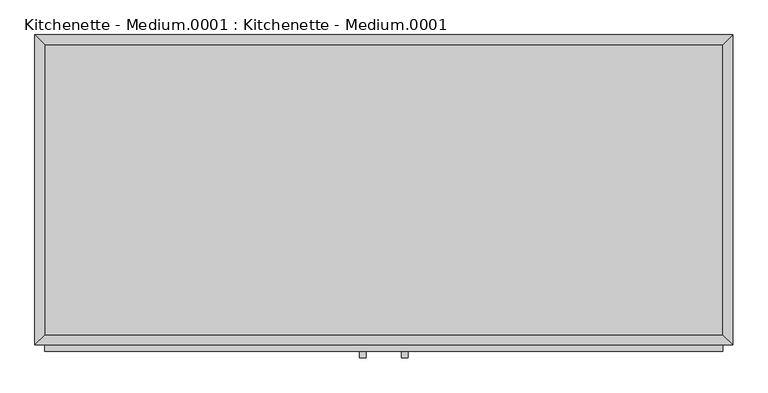
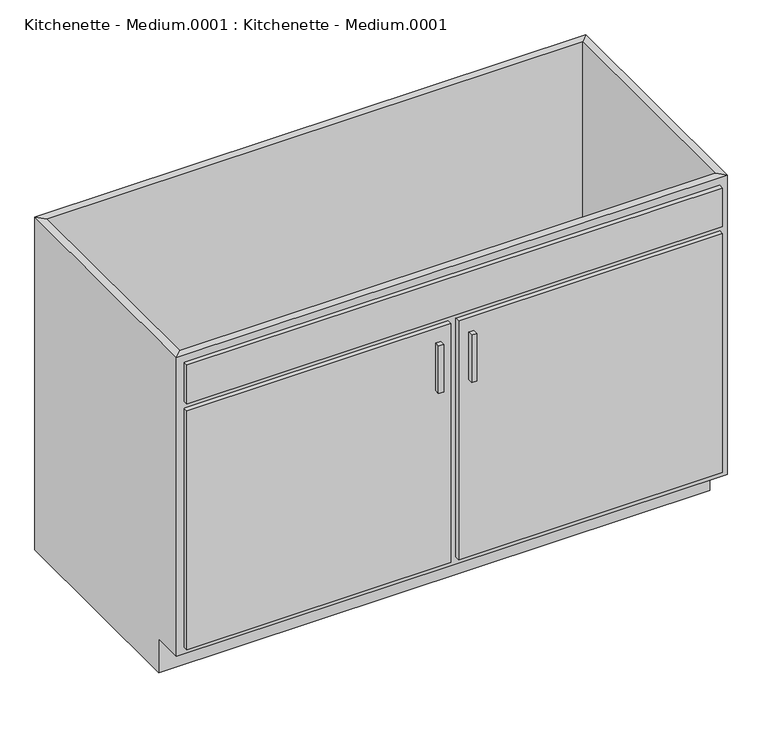
"""IFC4 building model written with IfcOpenShell, lengths in millimetres: proxy geometry, Kitchenette - Medium.0001 : Kitchenette - Medium.0001."""

from ifc_helpers import new_model, si_unit, frame, origin, place, context, project, spatial, polyline, outline, extrude, faceted_brep, source, transform, mapped, element, save


def kitchenette_medium_0001_kitchenette_medium_0001_844211aa(model_context):
    return source(origin(), model_context, "Body", "SolidModel", [
        faceted_brep([(685.4877049, -590.55, 876.3), (685.4877049, -590.55, 88.9), (-648.0122951, -590.55, 88.9), (-648.0122951, -590.55, 876.3), (-667.0622951, -609.6, 876.3), (704.5377049, -609.6, 876.3), (-667.0622951, -609.6, 88.9), (704.5377049, -609.6, 88.9), (-648.0122951, -533.4, 88.9), (-648.0122951, -19.05, 88.9), (-648.0122951, -19.05, 876.3), (-667.0622951, 0.0, 876.3), (-667.0622951, 0.0, 0.0), (-667.0622951, -533.4, 0.0), (-667.0622951, -533.4, 88.9), (685.4877049, -19.05, 88.9), (685.4877049, -19.05, 876.3), (704.5377049, 0.0, 876.3), (704.5377049, 0.0, 0.0), (685.4877049, -533.4, 88.9), (704.5377049, -533.4, 88.9), (704.5377049, -533.4, 0.0)], [[[0, 1, 2, 3]], [[0, 3, 4, 5]], [[5, 4, 6, 7]], [[2, 1, 7, 6]], [[3, 2, 8, 9, 10]], [[4, 3, 10, 11]], [[6, 4, 11, 12, 13, 14]], [[2, 6, 14, 8]], [[10, 9, 15, 16]], [[11, 10, 16, 17]], [[12, 11, 17, 18]], [[1, 0, 16, 15, 19]], [[0, 5, 17, 16]], [[5, 7, 20, 21, 18, 17]], [[7, 1, 19, 20]], [[8, 19, 15, 9]], [[18, 21, 13, 12]], [[13, 21, 20, 19, 8, 14]]]),
        extrude(outline(polyline([(-16.1872951, -635.0), (-28.8872951, -635.0), (-28.8872951, -622.3), (-16.1872951, -622.3), (-16.1872951, -635.0)])), frame((0.0, 0.0, 573.769895), z_axis=(0.0, 0.0, 1.0), x_axis=(1.0, 0.0, 0.0)), (0.0, 0.0, 1.0), 124.730105),
        extrude(outline(polyline([(66.3627049, -635.0), (53.6627049, -635.0), (53.6627049, -622.3), (66.3627049, -622.3), (66.3627049, -635.0)])), frame((0.0, 0.0, 573.769895), z_axis=(0.0, 0.0, 1.0), x_axis=(1.0, 0.0, 0.0)), (0.0, 0.0, 1.0), 124.730105),
        extrude(outline(polyline([(685.4877049, -19.05), (685.4877049, -590.55), (-648.0122951, -590.55), (-648.0122951, -19.05), (685.4877049, -19.05)])), frame((0.0, 0.0, 88.9), z_axis=(0.0, 0.0, 1.0), x_axis=(1.0, 0.0, 0.0)), (0.0, 0.0, 1.0), 19.05),
        extrude(outline(polyline([(9.2127049, -622.3), (-648.0122951, -622.3), (-648.0122951, -609.6), (9.2127049, -609.6), (9.2127049, -622.3)])), frame((0.0, 0.0, 107.95), z_axis=(0.0, 0.0, 1.0), x_axis=(1.0, 0.0, 0.0)), (0.0, 0.0, 1.0), 628.65),
        extrude(outline(polyline([(685.4877049, -622.3), (28.2627049, -622.3), (28.2627049, -609.6), (685.4877049, -609.6), (685.4877049, -622.3)])), frame((0.0, 0.0, 107.95), z_axis=(0.0, 0.0, 1.0), x_axis=(1.0, 0.0, 0.0)), (0.0, 0.0, 1.0), 628.65),
        extrude(outline(polyline([(685.4877049, -622.3), (-648.0122951, -622.3), (-648.0122951, -609.6), (685.4877049, -609.6), (685.4877049, -622.3)])), frame((0.0, 0.0, 755.65), z_axis=(0.0, 0.0, 1.0), x_axis=(1.0, 0.0, 0.0)), (0.0, 0.0, 1.0), 101.6),
    ])


if __name__ == "__main__":
    model = new_model("IFC4")
    model_context = context("Model", 3, world=origin())
    ifc_project = project(units=[si_unit("LENGTHUNIT", "METRE", prefix="MILLI")], contexts=[model_context])
    site = spatial("IfcSite", under=ifc_project)
    building = spatial("IfcBuilding", under=site)
    placement = place(None, origin())
    kitchenette_medium_0001_kitchenette_medium_0001_shape = kitchenette_medium_0001_kitchenette_medium_0001_844211aa(model_context)
    element("IfcBuildingElementProxy", 1, Name="Kitchenette - Medium.0001 : Kitchenette - Medium.0001", ObjectType="Kitchenette - Medium.0001 : Kitchenette - Medium.0001", at=placement, inside=building, context=model_context, shape_type="MappedRepresentation", body=[
        mapped(kitchenette_medium_0001_kitchenette_medium_0001_shape, transform((0.0, 0.0, 0.0), x_axis=(1.0, 0.0, 0.0), y_axis=(0.0, 1.0, 0.0), z_axis=(0.0, 0.0, 1.0))),
    ])
    save(model, "model.ifc")

# Revit data of these elements
# Type "Kitchenette - Medium.0001 : Kitchenette - Medium.0001"
#   Assembly Code = "E1090400"
#   Counter Length = 6' - 6"
#   Cabinet Width = 4' - 6"
#   Cabinet Height = 2' - 10 1/2"
#   Cabinet Depth = 2' - 0"
#   Toe Depth = 0' - 3"
#   Toe Height = 0' - 3 1/2"
#   Cabinet Material = Cabinets
#   Door/Drawer Material = Cabinets
#   Handle Material = Cabinets - Handles
#   Default Elevation = 0
# Element 1 (IfcBuildingElementProxy, "Kitchenette - Medium.0001 : Kitchenette - Medium.0001")
#   Materials on its faces: "Cabinets", "Cabinets - Handles"
# Materials
#   "Cabinets": colour RGB 249 249 249, transparency 0
#   "Cabinets - Handles": class "Metal", colour RGB 57 57 57, transparency 0
